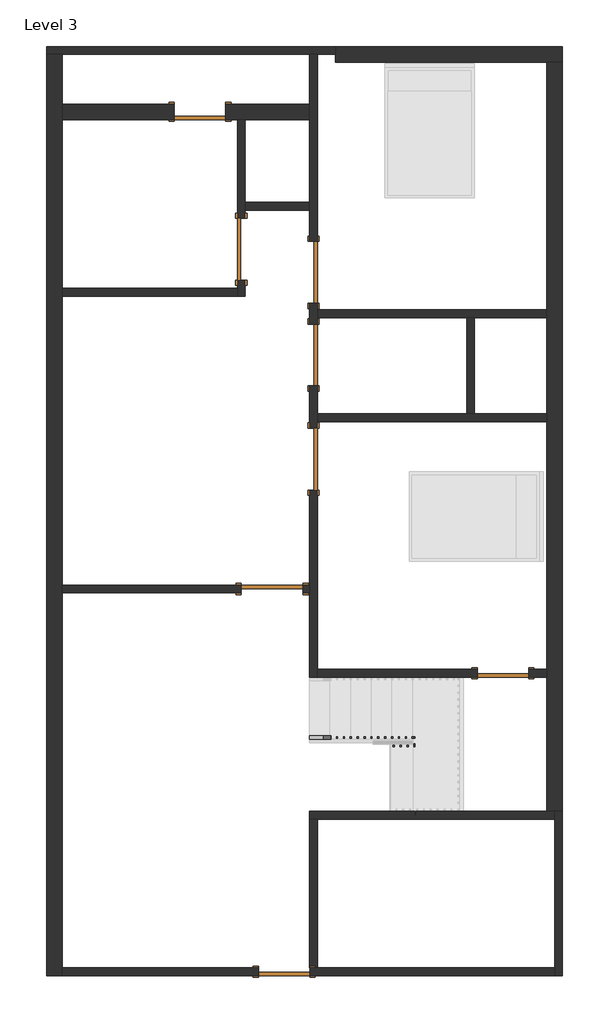
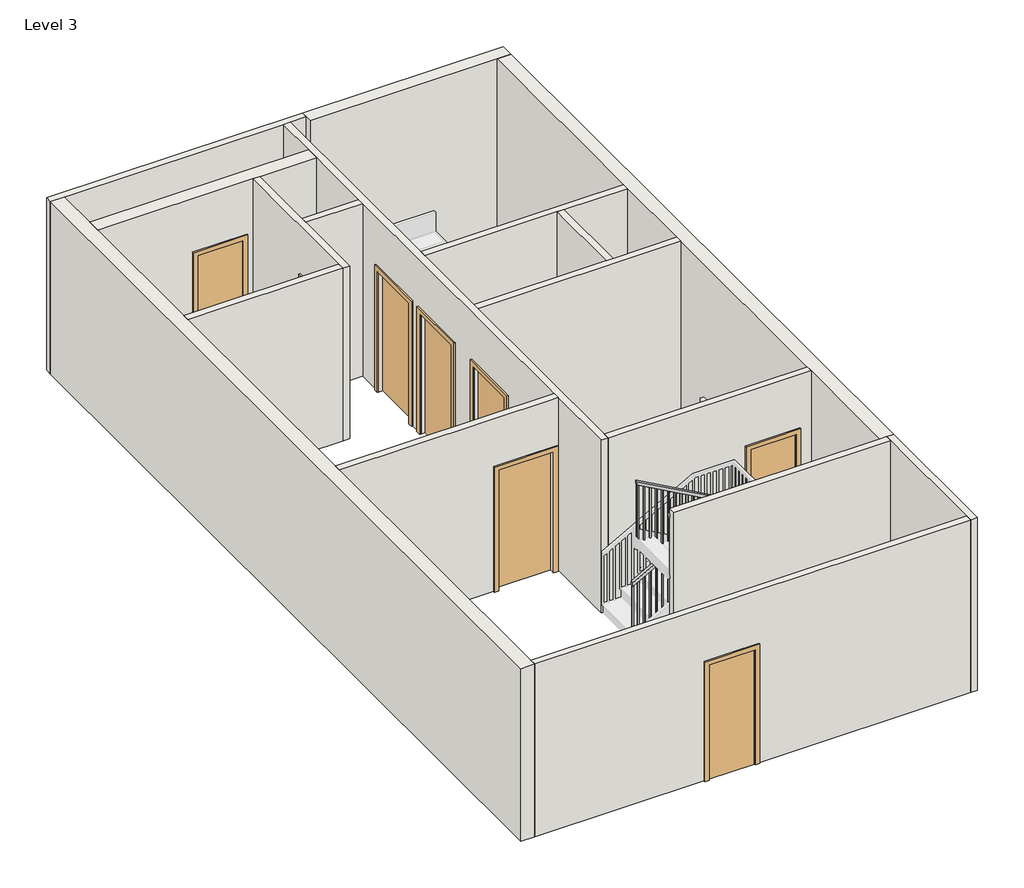
# One storey, part 1 of 2: 18 walls, 8 doors, 1 railing.
"""IFC4 building model written with IfcOpenShell, lengths in millimetres."""

from ifc_helpers import new_model, si_unit, frame, origin, place, context, project, spatial, polyline, outline, extrude, faceted_brep, transform, mapped, element, save
from components import door_85036156, door_d8f5dbb5, door_305aa2a5, door_e5f9f3c4

model = new_model("IFC4")

# Units and contexts
model_context = context("Model", 3, world=origin())
ifc_project = project(units=[si_unit("LENGTHUNIT", "METRE", prefix="MILLI")], contexts=[model_context])

# Site, building, storey
site = spatial("IfcSite", under=ifc_project)
building = spatial("IfcBuilding", under=site)
storey = spatial("IfcBuildingStorey", under=building, Name="Level 3", Elevation=3200.4)

# Doors
placement = place(None, origin())
door_shape = door_85036156(model_context)
element("IfcDoor", 1, ObjectType="Single-Flush : 30\" x 80\"", at=placement, inside=storey, context=model_context, shape_type="MappedRepresentation", body=[
    mapped(door_shape, transform((-2798.2915084, 6430.9935985, 3200.4), x_axis=(1.0, 0.0, 0.0), y_axis=(0.0, 1.0, 0.0), z_axis=(0.0, 0.0, 1.0))),
])
door_2_shape = door_d8f5dbb5(model_context)
element("IfcDoor", 2, ObjectType="Single-Flush : 30\" x 80\"", at=placement, inside=storey, context=model_context, shape_type="MappedRepresentation", body=[
    mapped(door_2_shape, transform((1678.4584916, -1855.7564015, 3200.4), x_axis=(-1.0, 0.0, 0.0), y_axis=(0.0, -1.0, 0.0), z_axis=(0.0, 0.0, 1.0))),
])
element("IfcDoor", 3, ObjectType="Single-Flush : 30\" x 80\"", at=placement, inside=storey, context=model_context, shape_type="MappedRepresentation", body=[
    mapped(door_2_shape, transform((-1553.6915084, -6262.6564015, 3200.4), x_axis=(-1.0, 0.0, 0.0), y_axis=(0.0, -1.0, 0.0), z_axis=(0.0, 0.0, 1.0))),
])
door_3_shape = door_305aa2a5(model_context)
element("IfcDoor", 4, ObjectType="Single-Flush : 36\" x 84\"", at=placement, inside=storey, context=model_context, shape_type="MappedRepresentation", body=[
    mapped(door_3_shape, transform((-2188.6915084, 4405.3435985, 3200.4), x_axis=(0.0, -1.0, 0.0), y_axis=(1.0, 0.0, 0.0), z_axis=(0.0, 0.0, 1.0))),
])
element("IfcDoor", 5, ObjectType="Single-Flush : 36\" x 84\"", at=placement, inside=storey, context=model_context, shape_type="MappedRepresentation", body=[
    mapped(door_3_shape, transform((-1121.8915084, 1306.5435985, 3200.4), x_axis=(0.0, 1.0, 0.0), y_axis=(-1.0, 0.0, 0.0), z_axis=(0.0, 0.0, 1.0))),
])
door_4_shape = door_e5f9f3c4(model_context)
element("IfcDoor", 6, ObjectType="Single-Flush : 36\" x 84\"", at=placement, inside=storey, context=model_context, shape_type="MappedRepresentation", body=[
    mapped(door_4_shape, transform((-1121.8915084, 4062.4435985, 3200.4), x_axis=(0.0, -1.0, 0.0), y_axis=(1.0, 0.0, 0.0), z_axis=(0.0, 0.0, 1.0))),
])
element("IfcDoor", 7, ObjectType="Single-Flush : 36\" x 84\"", at=placement, inside=storey, context=model_context, shape_type="MappedRepresentation", body=[
    mapped(door_4_shape, transform((-1121.8915084, 2843.2435985, 3200.4), x_axis=(0.0, -1.0, 0.0), y_axis=(1.0, 0.0, 0.0), z_axis=(0.0, 0.0, 1.0))),
])
element("IfcDoor", 8, ObjectType="Single-Flush : 36\" x 84\"", at=placement, inside=storey, context=model_context, shape_type="MappedRepresentation", body=[
    mapped(door_4_shape, transform((-1731.4915084, -611.1564015, 3200.4), x_axis=(1.0, 0.0, 0.0), y_axis=(0.0, 1.0, 0.0), z_axis=(0.0, 0.0, 1.0))),
])

# Railing
element("IfcRailing", 9, ObjectType="Handrail - Rectangular", at=placement, inside=storey, context=model_context, shape_type="SolidModel", body=[
    faceted_brep([(-1179.0415084, -2776.5064015, 4284.1333333), (-1179.0415084, -2776.5064015, 4226.020221), (-1179.0415084, -2827.3064015, 4226.020221), (-1179.0415084, -2827.3064015, 4284.1333333), (268.7584916, -2776.5064015, 5088.4666667), (319.5584916, -2776.5064015, 5058.5757765), (319.5584916, -2827.3064015, 5058.5757765), (268.7584916, -2827.3064015, 5088.4666667), (268.7584916, -2776.5064015, 5130.8), (319.5584916, -2776.5064015, 5080.0), (319.5584916, -2827.3064015, 5080.0), (268.7584916, -2827.3064015, 5130.8), (395.7584916, -2776.5064015, 5130.8), (395.7584916, -2776.5064015, 5080.0), (344.9584916, -2827.3064015, 5080.0), (344.9584916, -2827.3064015, 5130.8), (395.7584916, -2903.5064015, 5130.8), (395.7584916, -2903.5064015, 5080.0), (344.9584916, -2903.5064015, 5080.0), (344.9584916, -2903.5064015, 5130.8), (395.7584916, -2928.9064015, 5130.8), (344.9584916, -2928.9064015, 5130.8), (344.9584916, -2928.9064015, 5080.0), (395.7584916, -2928.9064015, 5080.0)], [[[0, 1, 2, 3]], [[1, 0, 4, 5]], [[2, 1, 5, 6]], [[3, 2, 6, 7]], [[0, 3, 7, 4]], [[5, 4, 8, 9]], [[6, 5, 9, 10]], [[7, 6, 10, 11]], [[4, 7, 11, 8]], [[9, 8, 12, 13]], [[10, 9, 13, 14]], [[11, 10, 14, 15]], [[8, 11, 15, 12]], [[13, 12, 16, 17]], [[14, 13, 17, 18]], [[15, 14, 18, 19]], [[12, 15, 19, 16]], [[20, 21, 22, 23]], [[17, 16, 20, 23]], [[18, 17, 23, 22]], [[19, 18, 22, 21]], [[16, 19, 21, 20]]]),
    faceted_brep([(395.7584916, -2903.5064015, 5130.8), (395.7584916, -2954.3064015, 5080.0), (344.9584916, -2954.3064015, 5080.0), (344.9584916, -2903.5064015, 5130.8), (395.7584916, -2903.5064015, 5271.9111111), (344.9584916, -2903.5064015, 5242.020221), (344.9584916, -2954.3064015, 5242.020221), (395.7584916, -2954.3064015, 5271.9111111)], [[[0, 1, 2, 3]], [[4, 5, 6, 7]], [[1, 0, 4, 7]], [[2, 1, 7, 6]], [[3, 2, 6, 5]], [[0, 3, 5, 4]]]),
    faceted_brep([(395.7584916, -2954.3064015, 5271.9111111), (344.9584916, -2954.3064015, 5242.020221), (344.9584916, -2903.5064015, 5242.020221), (395.7584916, -2903.5064015, 5271.9111111), (-1179.0415084, -2954.3064015, 6146.8), (-1179.0415084, -2903.5064015, 6146.8), (-1179.0415084, -2903.5064015, 6088.6868876), (-1179.0415084, -2954.3064015, 6088.6868876)], [[[0, 1, 2, 3]], [[4, 5, 6, 7]], [[1, 0, 4, 7]], [[2, 1, 7, 6]], [[3, 2, 6, 5]], [[0, 3, 5, 4]]]),
    extrude(outline(polyline([(6069.2841099, -1144.1165084), (6079.8674432, -1163.1665084), (5063.0666667, -1163.1665084), (5063.0666667, -1144.1165084), (6069.2841099, -1144.1165084)])), frame((0.0, -2938.4314015, 0.0), z_axis=(0.0, 1.0, 0.0), x_axis=(0.0, 0.0, 1.0)), (0.0, 0.0, 1.0), 19.05),
    extrude(outline(polyline([(6012.8396654, -1042.5165084), (6023.4229988, -1061.5665084), (5063.0666667, -1061.5665084), (5063.0666667, -1042.5165084), (6012.8396654, -1042.5165084)])), frame((0.0, -2938.4314015, 0.0), z_axis=(0.0, 1.0, 0.0), x_axis=(0.0, 0.0, 1.0)), (0.0, 0.0, 1.0), 19.05),
    extrude(outline(polyline([(5956.395221, -940.9165084), (5966.9785543, -959.9665084), (5063.0666667, -959.9665084), (5063.0666667, -940.9165084), (5956.395221, -940.9165084)])), frame((0.0, -2938.4314015, 0.0), z_axis=(0.0, 1.0, 0.0), x_axis=(0.0, 0.0, 1.0)), (0.0, 0.0, 1.0), 19.05),
    extrude(outline(polyline([(5899.9507765, -839.3165084), (5910.5341099, -858.3665084), (4893.7333333, -858.3665084), (4893.7333333, -839.3165084), (5899.9507765, -839.3165084)])), frame((0.0, -2938.4314015, 0.0), z_axis=(0.0, 1.0, 0.0), x_axis=(0.0, 0.0, 1.0)), (0.0, 0.0, 1.0), 19.05),
    extrude(outline(polyline([(5843.5063321, -737.7165084), (5854.0896654, -756.7665084), (4893.7333333, -756.7665084), (4893.7333333, -737.7165084), (5843.5063321, -737.7165084)])), frame((0.0, -2938.4314015, 0.0), z_axis=(0.0, 1.0, 0.0), x_axis=(0.0, 0.0, 1.0)), (0.0, 0.0, 1.0), 19.05),
    extrude(outline(polyline([(5787.0618876, -636.1165084), (5797.645221, -655.1665084), (4893.7333333, -655.1665084), (4893.7333333, -636.1165084), (5787.0618876, -636.1165084)])), frame((0.0, -2938.4314015, 0.0), z_axis=(0.0, 1.0, 0.0), x_axis=(0.0, 0.0, 1.0)), (0.0, 0.0, 1.0), 19.05),
    extrude(outline(polyline([(5730.6174432, -534.5165084), (5741.2007765, -553.5665084), (4724.4, -553.5665084), (4724.4, -534.5165084), (5730.6174432, -534.5165084)])), frame((0.0, -2938.4314015, 0.0), z_axis=(0.0, 1.0, 0.0), x_axis=(0.0, 0.0, 1.0)), (0.0, 0.0, 1.0), 19.05),
    extrude(outline(polyline([(5674.1729988, -432.9165084), (5684.7563321, -451.9665084), (4724.4, -451.9665084), (4724.4, -432.9165084), (5674.1729988, -432.9165084)])), frame((0.0, -2938.4314015, 0.0), z_axis=(0.0, 1.0, 0.0), x_axis=(0.0, 0.0, 1.0)), (0.0, 0.0, 1.0), 19.05),
    extrude(outline(polyline([(5617.7285543, -331.3165084), (5628.3118876, -350.3665084), (4724.4, -350.3665084), (4724.4, -331.3165084), (5617.7285543, -331.3165084)])), frame((0.0, -2938.4314015, 0.0), z_axis=(0.0, 1.0, 0.0), x_axis=(0.0, 0.0, 1.0)), (0.0, 0.0, 1.0), 19.05),
    extrude(outline(polyline([(5561.2841099, -229.7165084), (5571.8674432, -248.7665084), (4555.0666667, -248.7665084), (4555.0666667, -229.7165084), (5561.2841099, -229.7165084)])), frame((0.0, -2938.4314015, 0.0), z_axis=(0.0, 1.0, 0.0), x_axis=(0.0, 0.0, 1.0)), (0.0, 0.0, 1.0), 19.05),
    extrude(outline(polyline([(5504.8396654, -128.1165084), (5515.4229988, -147.1665084), (4555.0666667, -147.1665084), (4555.0666667, -128.1165084), (5504.8396654, -128.1165084)])), frame((0.0, -2938.4314015, 0.0), z_axis=(0.0, 1.0, 0.0), x_axis=(0.0, 0.0, 1.0)), (0.0, 0.0, 1.0), 19.05),
    extrude(outline(polyline([(5448.395221, -26.5165084), (5458.9785543, -45.5665084), (4555.0666667, -45.5665084), (4555.0666667, -26.5165084), (5448.395221, -26.5165084)])), frame((0.0, -2938.4314015, 0.0), z_axis=(0.0, 1.0, 0.0), x_axis=(0.0, 0.0, 1.0)), (0.0, 0.0, 1.0), 19.05),
    extrude(outline(polyline([(5391.9507765, 75.0834916), (5402.5341099, 56.0334916), (4385.7333333, 56.0334916), (4385.7333333, 75.0834916), (5391.9507765, 75.0834916)])), frame((0.0, -2938.4314015, 0.0), z_axis=(0.0, 1.0, 0.0), x_axis=(0.0, 0.0, 1.0)), (0.0, 0.0, 1.0), 19.05),
    extrude(outline(polyline([(5335.5063321, 176.6834916), (5346.0896654, 157.6334916), (4385.7333333, 157.6334916), (4385.7333333, 176.6834916), (5335.5063321, 176.6834916)])), frame((0.0, -2938.4314015, 0.0), z_axis=(0.0, 1.0, 0.0), x_axis=(0.0, 0.0, 1.0)), (0.0, 0.0, 1.0), 19.05),
    extrude(outline(polyline([(5279.0618876, 278.2834916), (5289.645221, 259.2334916), (4385.7333333, 259.2334916), (4385.7333333, 278.2834916), (5279.0618876, 278.2834916)])), frame((0.0, -2938.4314015, 0.0), z_axis=(0.0, 1.0, 0.0), x_axis=(0.0, 0.0, 1.0)), (0.0, 0.0, 1.0), 19.05),
    extrude(outline(polyline([(360.8334916, -2893.9814015), (379.8834916, -2893.9814015), (379.8834916, -2913.0314015), (360.8334916, -2913.0314015), (360.8334916, -2893.9814015)])), frame((0.0, 0.0, 4216.4), z_axis=(0.0, 0.0, 1.0), x_axis=(1.0, 0.0, 0.0)), (0.0, 0.0, 1.0), 863.6),
    extrude(outline(polyline([(335.4334916, -2811.4314015), (335.4334916, -2792.3814015), (354.4834916, -2792.3814015), (354.4834916, -2811.4314015), (335.4334916, -2811.4314015)])), frame((0.0, 0.0, 4216.4), z_axis=(0.0, 0.0, 1.0), x_axis=(1.0, 0.0, 0.0)), (0.0, 0.0, 1.0), 863.6),
    extrude(outline(polyline([(5021.5341099, 252.8834916), (5010.9507765, 233.8334916), (4047.0666667, 233.8334916), (4047.0666667, 252.8834916), (5021.5341099, 252.8834916)])), frame((0.0, -2811.4314015, 0.0), z_axis=(0.0, 1.0, 0.0), x_axis=(0.0, 0.0, 1.0)), (0.0, 0.0, 1.0), 19.05),
    extrude(outline(polyline([(4965.0896654, 151.2834916), (4954.5063321, 132.2334916), (4047.0666667, 132.2334916), (4047.0666667, 151.2834916), (4965.0896654, 151.2834916)])), frame((0.0, -2811.4314015, 0.0), z_axis=(0.0, 1.0, 0.0), x_axis=(0.0, 0.0, 1.0)), (0.0, 0.0, 1.0), 19.05),
    extrude(outline(polyline([(4908.645221, 49.6834916), (4898.0618876, 30.6334916), (4047.0666667, 30.6334916), (4047.0666667, 49.6834916), (4908.645221, 49.6834916)])), frame((0.0, -2811.4314015, 0.0), z_axis=(0.0, 1.0, 0.0), x_axis=(0.0, 0.0, 1.0)), (0.0, 0.0, 1.0), 19.05),
    extrude(outline(polyline([(4852.2007765, -51.9165084), (4841.6174432, -70.9665084), (3877.7333333, -70.9665084), (3877.7333333, -51.9165084), (4852.2007765, -51.9165084)])), frame((0.0, -2811.4314015, 0.0), z_axis=(0.0, 1.0, 0.0), x_axis=(0.0, 0.0, 1.0)), (0.0, 0.0, 1.0), 19.05),
    extrude(outline(polyline([(4795.7563321, -153.5165084), (4785.1729988, -172.5665084), (3877.7333333, -172.5665084), (3877.7333333, -153.5165084), (4795.7563321, -153.5165084)])), frame((0.0, -2811.4314015, 0.0), z_axis=(0.0, 1.0, 0.0), x_axis=(0.0, 0.0, 1.0)), (0.0, 0.0, 1.0), 19.05),
    extrude(outline(polyline([(4739.3118876, -255.1165084), (4728.7285543, -274.1665084), (3877.7333333, -274.1665084), (3877.7333333, -255.1165084), (4739.3118876, -255.1165084)])), frame((0.0, -2811.4314015, 0.0), z_axis=(0.0, 1.0, 0.0), x_axis=(0.0, 0.0, 1.0)), (0.0, 0.0, 1.0), 19.05),
    extrude(outline(polyline([(4682.8674432, -356.7165084), (4672.2841099, -375.7665084), (3708.4, -375.7665084), (3708.4, -356.7165084), (4682.8674432, -356.7165084)])), frame((0.0, -2811.4314015, 0.0), z_axis=(0.0, 1.0, 0.0), x_axis=(0.0, 0.0, 1.0)), (0.0, 0.0, 1.0), 19.05),
    extrude(outline(polyline([(4626.4229988, -458.3165084), (4615.8396654, -477.3665084), (3708.4, -477.3665084), (3708.4, -458.3165084), (4626.4229988, -458.3165084)])), frame((0.0, -2811.4314015, 0.0), z_axis=(0.0, 1.0, 0.0), x_axis=(0.0, 0.0, 1.0)), (0.0, 0.0, 1.0), 19.05),
    extrude(outline(polyline([(4569.9785543, -559.9165084), (4559.395221, -578.9665084), (3708.4, -578.9665084), (3708.4, -559.9165084), (4569.9785543, -559.9165084)])), frame((0.0, -2811.4314015, 0.0), z_axis=(0.0, 1.0, 0.0), x_axis=(0.0, 0.0, 1.0)), (0.0, 0.0, 1.0), 19.05),
    extrude(outline(polyline([(4513.5341099, -661.5165084), (4502.9507765, -680.5665084), (3539.0666667, -680.5665084), (3539.0666667, -661.5165084), (4513.5341099, -661.5165084)])), frame((0.0, -2811.4314015, 0.0), z_axis=(0.0, 1.0, 0.0), x_axis=(0.0, 0.0, 1.0)), (0.0, 0.0, 1.0), 19.05),
    extrude(outline(polyline([(4457.0896654, -763.1165084), (4446.5063321, -782.1665084), (3539.0666667, -782.1665084), (3539.0666667, -763.1165084), (4457.0896654, -763.1165084)])), frame((0.0, -2811.4314015, 0.0), z_axis=(0.0, 1.0, 0.0), x_axis=(0.0, 0.0, 1.0)), (0.0, 0.0, 1.0), 19.05),
    extrude(outline(polyline([(4400.645221, -864.7165084), (4390.0618876, -883.7665084), (3539.0666667, -883.7665084), (3539.0666667, -864.7165084), (4400.645221, -864.7165084)])), frame((0.0, -2811.4314015, 0.0), z_axis=(0.0, 1.0, 0.0), x_axis=(0.0, 0.0, 1.0)), (0.0, 0.0, 1.0), 19.05),
    extrude(outline(polyline([(4344.2007765, -966.3165084), (4333.6174432, -985.3665084), (3369.7333333, -985.3665084), (3369.7333333, -966.3165084), (4344.2007765, -966.3165084)])), frame((0.0, -2811.4314015, 0.0), z_axis=(0.0, 1.0, 0.0), x_axis=(0.0, 0.0, 1.0)), (0.0, 0.0, 1.0), 19.05),
    extrude(outline(polyline([(4287.7563321, -1067.9165084), (4277.1729988, -1086.9665084), (3369.7333333, -1086.9665084), (3369.7333333, -1067.9165084), (4287.7563321, -1067.9165084)])), frame((0.0, -2811.4314015, 0.0), z_axis=(0.0, 1.0, 0.0), x_axis=(0.0, 0.0, 1.0)), (0.0, 0.0, 1.0), 19.05),
    extrude(outline(polyline([(360.8334916, -2919.3814015), (379.8834916, -2919.3814015), (379.8834916, -2938.4314015), (360.8334916, -2938.4314015), (360.8334916, -2919.3814015)])), frame((0.0, 0.0, 4216.4), z_axis=(0.0, 0.0, 1.0), x_axis=(1.0, 0.0, 0.0)), (0.0, 0.0, 1.0), 863.6),
    extrude(outline(polyline([(360.8334916, -2811.4314015), (360.8334916, -2792.3814015), (379.8834916, -2792.3814015), (379.8834916, -2811.4314015), (360.8334916, -2811.4314015)])), frame((0.0, 0.0, 4216.4), z_axis=(0.0, 0.0, 1.0), x_axis=(1.0, 0.0, 0.0)), (0.0, 0.0, 1.0), 863.6),
    extrude(outline(polyline([(6078.1035543, -1159.9915084), (6088.6868876, -1179.0415084), (5063.0666667, -1179.0415084), (5063.0666667, -1159.9915084), (6078.1035543, -1159.9915084)])), frame((0.0, -2938.4314015, 0.0), z_axis=(0.0, 1.0, 0.0), x_axis=(0.0, 0.0, 1.0)), (0.0, 0.0, 1.0), 19.05),
    extrude(outline(polyline([(4236.6035543, -1159.9915084), (4226.020221, -1179.0415084), (3369.7333333, -1179.0415084), (3369.7333333, -1159.9915084), (4236.6035543, -1159.9915084)])), frame((0.0, -2811.4314015, 0.0), z_axis=(0.0, 1.0, 0.0), x_axis=(0.0, 0.0, 1.0)), (0.0, 0.0, 1.0), 19.05),
])

# Walls
element("IfcWall", 10, ObjectType="WALL 9\"", at=placement, inside=storey, context=model_context, shape_type="Brep", body=[
    faceted_brep([(-798.0415084, 7167.5935985, 3200.4), (2326.1584916, 7167.5935985, 3200.4), (2554.7584916, 7167.5935985, 3200.4), (2554.7584916, 7167.5935985, 6248.4), (2326.1584916, 7167.5935985, 6248.4), (-798.0415084, 7167.5935985, 6248.4), (-798.0415084, 7396.1935985, 3200.4), (-798.0415084, 7396.1935985, 6248.4), (2554.7584916, 7396.1935985, 6248.4), (2554.7584916, 7396.1935985, 3200.4), (-798.0415084, 7281.8935985, 3200.4), (-798.0415084, 7281.8935985, 6248.4)], [[[0, 1, 2, 3, 4, 5]], [[6, 7, 8, 9]], [[2, 1, 0, 10, 6, 9]], [[0, 5, 11, 7, 6, 10]], [[3, 2, 9, 8]], [[5, 4, 3, 8, 7, 11]]]),
])
element("IfcWall", 11, ObjectType="WALL 9\"", at=placement, inside=storey, context=model_context, shape_type="Brep", body=[
    faceted_brep([(2326.1584916, 7167.5935985, 3200.4), (2326.1584916, 3509.9935985, 3200.4), (2326.1584916, 3395.6935985, 3200.4), (2326.1584916, 1973.2935985, 3200.4), (2326.1584916, 1858.9935985, 3200.4), (2326.1584916, -1798.6064015, 3200.4), (2326.1584916, -1912.9064015, 3200.4), (2326.1584916, -3894.1064015, 3200.4), (2326.1584916, -3894.1064015, 6248.4), (2326.1584916, -1912.9064015, 6248.4), (2326.1584916, -1798.6064015, 6248.4), (2326.1584916, 1858.9935985, 6248.4), (2326.1584916, 1973.2935985, 6248.4), (2326.1584916, 3395.6935985, 6248.4), (2326.1584916, 3509.9935985, 6248.4), (2326.1584916, 7167.5935985, 6248.4), (2554.7584916, 7167.5935985, 3200.4), (2554.7584916, 7167.5935985, 6248.4), (2554.7584916, -3894.1064015, 6248.4), (2554.7584916, -3894.1064015, 3200.4), (2440.4584916, -3894.1064015, 3200.4), (2440.4584916, -3894.1064015, 6248.4)], [[[0, 1, 2, 3, 4, 5, 6, 7, 8, 9, 10, 11, 12, 13, 14, 15]], [[16, 17, 18, 19]], [[7, 6, 5, 4, 3, 2, 1, 0, 16, 19, 20]], [[0, 15, 17, 16]], [[8, 7, 20, 19, 18, 21]], [[15, 14, 13, 12, 11, 10, 9, 8, 21, 18, 17]]]),
])
element("IfcWall", 12, ObjectType="WALL 9\"", at=placement, inside=storey, context=model_context, shape_type="Brep", body=[
    faceted_brep([(-5065.2415084, 7281.8935985, 3200.4), (-5065.2415084, -6319.8064015, 3200.4), (-5065.2415084, -6319.8064015, 6248.4), (-5065.2415084, 7281.8935985, 6248.4), (-4836.6415084, 7281.8935985, 3200.4), (-4836.6415084, 7281.8935985, 6248.4), (-4836.6415084, 6545.2935985, 6248.4), (-4836.6415084, 6316.6935985, 6248.4), (-4836.6415084, 3827.4935985, 6248.4), (-4836.6415084, 3713.1935985, 6248.4), (-4836.6415084, -554.0064015, 6248.4), (-4836.6415084, -668.3064015, 6248.4), (-4836.6415084, -6205.5064015, 6248.4), (-4836.6415084, -6319.8064015, 6248.4), (-4836.6415084, -6319.8064015, 3200.4), (-4836.6415084, -6205.5064015, 3200.4), (-4836.6415084, -668.3064015, 3200.4), (-4836.6415084, -554.0064015, 3200.4), (-4836.6415084, 3713.1935985, 3200.4), (-4836.6415084, 3827.4935985, 3200.4), (-4836.6415084, 6316.6935985, 3200.4), (-4836.6415084, 6545.2935985, 3200.4)], [[[0, 1, 2, 3]], [[4, 5, 6, 7, 8, 9, 10, 11, 12, 13, 14, 15, 16, 17, 18, 19, 20, 21]], [[1, 0, 4, 21, 20, 19, 18, 17, 16, 15, 14]], [[0, 3, 5, 4]], [[3, 2, 13, 12, 11, 10, 9, 8, 7, 6, 5]], [[2, 1, 14, 13]]]),
])
element("IfcWall", 13, ObjectType="WALL 9\"", at=placement, inside=storey, context=model_context, shape_type="Brep", body=[
    faceted_brep([(-2417.2915084, 6316.6935985, 5232.4), (-2417.2915084, 6316.6935985, 3200.4), (-2245.8415084, 6316.6935985, 3200.4), (-2131.5415084, 6316.6935985, 3200.4), (-1179.0415084, 6316.6935985, 3200.4), (-1179.0415084, 6316.6935985, 6248.4), (-2131.5415084, 6316.6935985, 6248.4), (-2245.8415084, 6316.6935985, 6248.4), (-4836.6415084, 6316.6935985, 6248.4), (-4836.6415084, 6316.6935985, 3200.4), (-3179.2915084, 6316.6935985, 3200.4), (-3179.2915084, 6316.6935985, 5232.4), (-1179.0415084, 6545.2935985, 3200.4), (-2417.2915084, 6545.2935985, 3200.4), (-2417.2915084, 6545.2935985, 5232.4), (-3179.2915084, 6545.2935985, 5232.4), (-3179.2915084, 6545.2935985, 3200.4), (-4836.6415084, 6545.2935985, 3200.4), (-4836.6415084, 6545.2935985, 6248.4), (-1179.0415084, 6545.2935985, 6248.4)], [[[0, 1, 2, 3, 4, 5, 6, 7, 8, 9, 10, 11]], [[12, 13, 14, 15, 16, 17, 18, 19]], [[10, 9, 17, 16]], [[4, 3, 2, 1, 13, 12]], [[9, 8, 18, 17]], [[5, 4, 12, 19]], [[14, 13, 1, 0]], [[15, 14, 0, 11]], [[16, 15, 11, 10]], [[8, 7, 6, 5, 19, 18]]]),
])
element("IfcWall", 14, ObjectType="WALL4.5\"", at=placement, inside=storey, context=model_context, shape_type="Brep", body=[
    faceted_brep([(-5065.2415084, 7281.8935985, 3200.4), (-4836.6415084, 7281.8935985, 3200.4), (-1179.0415084, 7281.8935985, 3200.4), (-1064.7415084, 7281.8935985, 3200.4), (-798.0415084, 7281.8935985, 3200.4), (-798.0415084, 7281.8935985, 6248.4), (-1064.7415084, 7281.8935985, 6248.4), (-1179.0415084, 7281.8935985, 6248.4), (-4836.6415084, 7281.8935985, 6248.4), (-5065.2415084, 7281.8935985, 6248.4), (-5065.2415084, 7396.1935985, 3200.4), (-5065.2415084, 7396.1935985, 6248.4), (-798.0415084, 7396.1935985, 6248.4), (-798.0415084, 7396.1935985, 3200.4)], [[[0, 1, 2, 3, 4, 5, 6, 7, 8, 9]], [[10, 11, 12, 13]], [[4, 3, 2, 1, 0, 10, 13]], [[5, 4, 13, 12]], [[0, 9, 11, 10]], [[9, 8, 7, 6, 5, 12, 11]]]),
])
element("IfcWall", 15, ObjectType="WALL4.5\"", at=placement, inside=storey, context=model_context, shape_type="Brep", body=[
    faceted_brep([(2554.7584916, -6319.8064015, 3200.4), (2554.7584916, -3894.1064015, 3200.4), (2554.7584916, -3894.1064015, 6248.4), (2554.7584916, -6319.8064015, 6248.4), (2440.4584916, -6319.8064015, 3200.4), (2440.4584916, -6319.8064015, 6248.4), (2440.4584916, -6205.5064015, 6248.4), (2440.4584916, -4008.4064015, 6248.4), (2440.4584916, -3894.1064015, 6248.4), (2440.4584916, -3894.1064015, 3200.4), (2440.4584916, -4008.4064015, 3200.4), (2440.4584916, -6205.5064015, 3200.4)], [[[0, 1, 2, 3]], [[4, 5, 6, 7, 8, 9, 10, 11]], [[1, 0, 4, 11, 10, 9]], [[3, 2, 8, 7, 6, 5]], [[2, 1, 9, 8]], [[0, 3, 5, 4]]]),
])
element("IfcWall", 16, ObjectType="WALL4.5\"", at=placement, inside=storey, context=model_context, shape_type="Brep", body=[
    faceted_brep([(2440.4584916, -3894.1064015, 3200.4), (2326.1584916, -3894.1064015, 3200.4), (-1179.0415084, -3894.1064015, 3200.4), (-1179.0415084, -3894.1064015, 6248.4), (2326.1584916, -3894.1064015, 6248.4), (2440.4584916, -3894.1064015, 6248.4), (2440.4584916, -4008.4064015, 3200.4), (2440.4584916, -4008.4064015, 6248.4), (-1179.0415084, -4008.4064015, 6248.4), (-1179.0415084, -4008.4064015, 4419.6), (-1179.0415084, -4008.4064015, 3200.4), (-1064.7415084, -4008.4064015, 3200.4)], [[[0, 1, 2, 3, 4, 5]], [[6, 7, 8, 9, 10, 11]], [[2, 1, 0, 6, 11, 10]], [[0, 5, 7, 6]], [[3, 2, 10, 9, 8]], [[5, 4, 3, 8, 7]]]),
])
element("IfcWall", 17, ObjectType="WALL4.5\"", at=placement, inside=storey, context=model_context, shape_type="Brep", body=[
    faceted_brep([(-2245.8415084, 3948.1435985, 5334.0), (-2245.8415084, 3948.1435985, 3200.4), (-2245.8415084, 3827.4935985, 3200.4), (-2245.8415084, 3713.1935985, 3200.4), (-2245.8415084, 3713.1935985, 6248.4), (-2245.8415084, 3827.4935985, 6248.4), (-2245.8415084, 6316.6935985, 6248.4), (-2245.8415084, 6316.6935985, 3200.4), (-2245.8415084, 4862.5435985, 3200.4), (-2245.8415084, 4862.5435985, 5334.0), (-2131.5415084, 3713.1935985, 3200.4), (-2131.5415084, 3948.1435985, 3200.4), (-2131.5415084, 3948.1435985, 5334.0), (-2131.5415084, 4862.5435985, 5334.0), (-2131.5415084, 4862.5435985, 3200.4), (-2131.5415084, 4983.1935985, 3200.4), (-2131.5415084, 5097.4935985, 3200.4), (-2131.5415084, 6316.6935985, 3200.4), (-2131.5415084, 6316.6935985, 6248.4), (-2131.5415084, 5097.4935985, 6248.4), (-2131.5415084, 4983.1935985, 6248.4), (-2131.5415084, 3713.1935985, 6248.4)], [[[0, 1, 2, 3, 4, 5, 6, 7, 8, 9]], [[10, 11, 12, 13, 14, 15, 16, 17, 18, 19, 20, 21]], [[8, 7, 17, 16, 15, 14]], [[3, 2, 1, 11, 10]], [[7, 6, 18, 17]], [[4, 3, 10, 21]], [[12, 11, 1, 0]], [[13, 12, 0, 9]], [[14, 13, 9, 8]], [[6, 5, 4, 21, 20, 19, 18]]]),
])
element("IfcWall", 18, ObjectType="WALL4.5\"", at=placement, inside=storey, context=model_context, shape_type="SweptSolid", body=[
    extrude(outline(polyline([(-2245.8415084, 3713.1935985), (-4836.6415084, 3713.1935985), (-4836.6415084, 3827.4935985), (-2245.8415084, 3827.4935985), (-2245.8415084, 3713.1935985)])), frame((0.0, 0.0, 3200.4), z_axis=(0.0, 0.0, 1.0), x_axis=(1.0, 0.0, 0.0)), (0.0, 0.0, 1.0), 3048.0),
])
element("IfcWall", 19, ObjectType="WALL4.5\"", at=placement, inside=storey, context=model_context, shape_type="SweptSolid", body=[
    extrude(outline(polyline([(-1179.0415084, 4983.1935985), (-2131.5415084, 4983.1935985), (-2131.5415084, 5097.4935985), (-1179.0415084, 5097.4935985), (-1179.0415084, 4983.1935985)])), frame((0.0, 0.0, 3200.4), z_axis=(0.0, 0.0, 1.0), x_axis=(1.0, 0.0, 0.0)), (0.0, 0.0, 1.0), 3048.0),
])
element("IfcWall", 20, ObjectType="WALL4.5\"", at=placement, inside=storey, context=model_context, shape_type="Brep", body=[
    faceted_brep([(-1179.0415084, 2386.0435985, 3200.4), (-1179.0415084, 1763.7435985, 3200.4), (-1179.0415084, 1763.7435985, 5334.0), (-1179.0415084, 849.3435985, 5334.0), (-1179.0415084, 849.3435985, 3200.4), (-1179.0415084, -554.0064015, 3200.4), (-1179.0415084, -668.3064015, 3200.4), (-1179.0415084, -1912.9064015, 3200.4), (-1179.0415084, -1912.9064015, 6248.4), (-1179.0415084, -668.3064015, 6248.4), (-1179.0415084, -554.0064015, 6248.4), (-1179.0415084, 4983.1935985, 6248.4), (-1179.0415084, 5097.4935985, 6248.4), (-1179.0415084, 6316.6935985, 6248.4), (-1179.0415084, 6545.2935985, 6248.4), (-1179.0415084, 7281.8935985, 6248.4), (-1179.0415084, 7281.8935985, 3200.4), (-1179.0415084, 6545.2935985, 3200.4), (-1179.0415084, 6316.6935985, 3200.4), (-1179.0415084, 5097.4935985, 3200.4), (-1179.0415084, 4983.1935985, 3200.4), (-1179.0415084, 4519.6435985, 3200.4), (-1179.0415084, 4519.6435985, 5334.0), (-1179.0415084, 3605.2435985, 5334.0), (-1179.0415084, 3605.2435985, 3200.4), (-1179.0415084, 3300.4435985, 3200.4), (-1179.0415084, 3300.4435985, 5334.0), (-1179.0415084, 2386.0435985, 5334.0), (-1064.7415084, 1763.7435985, 5334.0), (-1064.7415084, 1763.7435985, 3200.4), (-1064.7415084, 1858.9935985, 3200.4), (-1064.7415084, 1973.2935985, 3200.4), (-1064.7415084, 2386.0435985, 3200.4), (-1064.7415084, 2386.0435985, 5334.0), (-1064.7415084, 3300.4435985, 5334.0), (-1064.7415084, 3300.4435985, 3200.4), (-1064.7415084, 3395.6935985, 3200.4), (-1064.7415084, 3509.9935985, 3200.4), (-1064.7415084, 3605.2435985, 3200.4), (-1064.7415084, 3605.2435985, 5334.0), (-1064.7415084, 4519.6435985, 5334.0), (-1064.7415084, 4519.6435985, 3200.4), (-1064.7415084, 7281.8935985, 3200.4), (-1064.7415084, 7281.8935985, 6248.4), (-1064.7415084, 3509.9935985, 6248.4), (-1064.7415084, 3395.6935985, 6248.4), (-1064.7415084, 1973.2935985, 6248.4), (-1064.7415084, 1858.9935985, 6248.4), (-1064.7415084, -1798.6064015, 6248.4), (-1064.7415084, -1912.9064015, 6248.4), (-1064.7415084, -1912.9064015, 3200.4), (-1064.7415084, -1798.6064015, 3200.4), (-1064.7415084, 849.3435985, 3200.4), (-1064.7415084, 849.3435985, 5334.0)], [[[0, 1, 2, 3, 4, 5, 6, 7, 8, 9, 10, 11, 12, 13, 14, 15, 16, 17, 18, 19, 20, 21, 22, 23, 24, 25, 26, 27]], [[28, 29, 30, 31, 32, 33, 34, 35, 36, 37, 38, 39, 40, 41, 42, 43, 44, 45, 46, 47, 48, 49, 50, 51, 52, 53]], [[21, 20, 19, 18, 17, 16, 42, 41]], [[25, 24, 38, 37, 36, 35]], [[52, 51, 50, 7, 6, 5, 4]], [[32, 31, 30, 29, 1, 0]], [[16, 15, 43, 42]], [[8, 7, 50, 49]], [[39, 38, 24, 23]], [[40, 39, 23, 22]], [[41, 40, 22, 21]], [[33, 32, 0, 27]], [[34, 33, 27, 26]], [[35, 34, 26, 25]], [[2, 1, 29, 28]], [[3, 2, 28, 53]], [[4, 3, 53, 52]], [[15, 14, 13, 12, 11, 10, 9, 8, 49, 48, 47, 46, 45, 44, 43]]]),
])
element("IfcWall", 21, ObjectType="WALL4.5\"", at=placement, inside=storey, context=model_context, shape_type="SweptSolid", body=[
    extrude(outline(polyline([(3200.4, -1064.7415084), (3200.4, 1297.4584916), (5232.4, 1297.4584916), (5232.4, 2059.4584916), (3200.4, 2059.4584916), (3200.4, 2326.1584916), (6248.4, 2326.1584916), (6248.4, -1064.7415084), (3200.4, -1064.7415084)])), frame((0.0, -1912.9064015, 0.0), z_axis=(0.0, 1.0, 0.0), x_axis=(0.0, 0.0, 1.0)), (0.0, 0.0, 1.0), 114.3),
])
element("IfcWall", 22, ObjectType="WALL4.5\"", at=placement, inside=storey, context=model_context, shape_type="Brep", body=[
    faceted_brep([(-1064.7415084, 3395.6935985, 3200.4), (1145.0584916, 3395.6935985, 3200.4), (1259.3584916, 3395.6935985, 3200.4), (2326.1584916, 3395.6935985, 3200.4), (2326.1584916, 3395.6935985, 6248.4), (1259.3584916, 3395.6935985, 6248.4), (1145.0584916, 3395.6935985, 6248.4), (-1064.7415084, 3395.6935985, 6248.4), (-1064.7415084, 3509.9935985, 3200.4), (-1064.7415084, 3509.9935985, 6248.4), (2326.1584916, 3509.9935985, 6248.4), (2326.1584916, 3509.9935985, 3200.4)], [[[0, 1, 2, 3, 4, 5, 6, 7]], [[8, 9, 10, 11]], [[3, 2, 1, 0, 8, 11]], [[4, 3, 11, 10]], [[0, 7, 9, 8]], [[7, 6, 5, 4, 10, 9]]]),
])
element("IfcWall", 23, ObjectType="WALL4.5\"", at=placement, inside=storey, context=model_context, shape_type="SweptSolid", body=[
    extrude(outline(polyline([(1259.3584916, 3395.6935985), (1259.3584916, 1973.2935985), (1145.0584916, 1973.2935985), (1145.0584916, 3395.6935985), (1259.3584916, 3395.6935985)])), frame((0.0, 0.0, 3200.4), z_axis=(0.0, 0.0, 1.0), x_axis=(1.0, 0.0, 0.0)), (0.0, 0.0, 1.0), 3048.0),
])
element("IfcWall", 24, ObjectType="WALL4.5\"", at=placement, inside=storey, context=model_context, shape_type="Brep", body=[
    faceted_brep([(-1064.7415084, 1858.9935985, 3200.4), (2326.1584916, 1858.9935985, 3200.4), (2326.1584916, 1858.9935985, 6248.4), (-1064.7415084, 1858.9935985, 6248.4), (-1064.7415084, 1973.2935985, 3200.4), (-1064.7415084, 1973.2935985, 6248.4), (1145.0584916, 1973.2935985, 6248.4), (1259.3584916, 1973.2935985, 6248.4), (2326.1584916, 1973.2935985, 6248.4), (2326.1584916, 1973.2935985, 3200.4), (1259.3584916, 1973.2935985, 3200.4), (1145.0584916, 1973.2935985, 3200.4)], [[[0, 1, 2, 3]], [[4, 5, 6, 7, 8, 9, 10, 11]], [[1, 0, 4, 11, 10, 9]], [[2, 1, 9, 8]], [[0, 3, 5, 4]], [[3, 2, 8, 7, 6, 5]]]),
])
element("IfcWall", 25, ObjectType="WALL4.5\"", at=placement, inside=storey, context=model_context, shape_type="SweptSolid", body=[
    extrude(outline(polyline([(5334.0, -1274.2915084), (3200.4, -1274.2915084), (3200.4, -1179.0415084), (6248.4, -1179.0415084), (6248.4, -4836.6415084), (3200.4, -4836.6415084), (3200.4, -2188.6915084), (5334.0, -2188.6915084), (5334.0, -1274.2915084)])), frame((0.0, -668.3064015, 0.0), z_axis=(0.0, 1.0, 0.0), x_axis=(0.0, 0.0, 1.0)), (0.0, 0.0, 1.0), 114.3),
])
element("IfcWall", 26, ObjectType="WALL4.5\"", at=placement, inside=storey, context=model_context, shape_type="SweptSolid", body=[
    extrude(outline(polyline([(-1179.0415084, -6205.5064015), (-1179.0415084, -4008.4064015), (-1064.7415084, -4008.4064015), (-1064.7415084, -6205.5064015), (-1179.0415084, -6205.5064015)])), frame((0.0, 0.0, 3200.4), z_axis=(0.0, 0.0, 1.0), x_axis=(1.0, 0.0, 0.0)), (0.0, 0.0, 1.0), 1219.2),
])
element("IfcWall", 27, ObjectType="WALL4.5\"", at=placement, inside=storey, context=model_context, shape_type="Brep", body=[
    faceted_brep([(-4836.6415084, -6319.8064015, 3200.4), (-1934.6915084, -6319.8064015, 3200.4), (-1934.6915084, -6319.8064015, 5232.4), (-1172.6915084, -6319.8064015, 5232.4), (-1172.6915084, -6319.8064015, 3200.4), (2440.4584916, -6319.8064015, 3200.4), (2440.4584916, -6319.8064015, 6248.4), (-4836.6415084, -6319.8064015, 6248.4), (-1934.6915084, -6205.5064015, 5232.4), (-1934.6915084, -6205.5064015, 3200.4), (-4836.6415084, -6205.5064015, 3200.4), (-4836.6415084, -6205.5064015, 6248.4), (2440.4584916, -6205.5064015, 6248.4), (2440.4584916, -6205.5064015, 3200.4), (-1064.7415084, -6205.5064015, 3200.4), (-1172.6915084, -6205.5064015, 3200.4), (-1172.6915084, -6205.5064015, 5232.4)], [[[0, 1, 2, 3, 4, 5, 6, 7]], [[8, 9, 10, 11, 12, 13, 14, 15, 16]], [[10, 9, 1, 0]], [[15, 14, 13, 5, 4]], [[7, 6, 12, 11]], [[0, 7, 11, 10]], [[6, 5, 13, 12]], [[2, 1, 9, 8]], [[3, 2, 8, 16]], [[4, 3, 16, 15]]]),
])

save(model, "model.ifc")

# Revit data of these elements
# Type "Single-Flush : 30\" x 80\""
#   Type Mark = "5"
#   Construction Type Id = "MDOOR"
#   Assembly Code = "C1020"
#   Analytic Construction = "Metal"
#   Thickness = 0' - 2"
#   Heat Transfer Coefficient (U) = 0.651978 BTU/(h·ft²·°F)
#   Height = 6' - 8"
#   Trim Projection Ext = 0' - 1"
#   Trim Projection Int = 0' - 1"
#   Trim Width = 0' - 3"
#   Width = 2' - 6"
#   Define Thermal Properties by = 1
#   Define Thermal Properties by = 1
#   Door Material = Door - Panel
#   Frame Material = Door - Frame
#   Visual Light Transmittance = 0
#   Solar Heat Gain Coefficient = 0
#   Function = (empty or 0)
#   Wall Closure = (empty or 0)
# Type "Single-Flush : 36\" x 84\""
#   Type Mark = "1"
#   Construction Type Id = "MDOOR"
#   Assembly Code = "C1020"
#   Analytic Construction = "Metal"
#   Thickness = 0' - 2"
#   Heat Transfer Coefficient (U) = 0.651978 BTU/(h·ft²·°F)
#   Height = 7' - 0"
#   Trim Projection Ext = 0' - 1"
#   Trim Projection Int = 0' - 1"
#   Trim Width = 0' - 3"
#   Width = 3' - 0"
#   Define Thermal Properties by = 1
#   Define Thermal Properties by = 1
#   Door Material = Door - Panel
#   Frame Material = Door - Frame
#   Visual Light Transmittance = 0
#   Solar Heat Gain Coefficient = 0
#   Function = (empty or 0)
#   Wall Closure = (empty or 0)
# Type "Handrail - Rectangular"
#   Assembly Code = "C2010400"
#   built-in parameter 1008612 = 0.0416667 (stored number, unit not read)
#   built-in parameter 1008611 = 0.0416667 (stored number, unit not read)
#   built-in parameter 1008609 = 0.333333 (stored number, unit not read)
#   built-in parameter 1008604 = 0.166667 (stored number, unit not read)
#   built-in parameter 1008603 = 0.166667 (stored number, unit not read)
#   Railing Height = 3' - 0"
#   built-in parameter 1008630 = 2
#   built-in parameter 1008610 = 2
#   built-in parameter 1008618 = Baluster - Square : 3/4"
# Type "WALL 9\""
#   Assembly Code = "B2010"
#   Layers, outside or top first: 0' - 9" no material (function 1)
# Type "WALL4.5\""
#   Assembly Code = "B2010"
#   Layers, outside or top first: 0' - 4 1/2" no material (function 1)
# Elements 1, 2, 3 (IfcDoor, "Single-Flush : 30\" x 80\"")
#   Phase Created = New Construction
#   Materials on its faces: "Door - Frame", "Door - Panel"
# Elements 4, 5, 6, 7, 8 (IfcDoor, "Single-Flush : 36\" x 84\"")
#   Phase Created = New Construction
#   Materials on its faces: "Door - Frame", "Door - Panel"
# Element 9 (IfcRailing, "Handrail - Rectangular")
#   Phase Created = New Construction
# Elements 10, 11, 12 (IfcWall, "WALL 9\"")
#   Top Offset = 0' - 0"
#   Base Offset = 0' - 0"
#   Unconnected Height = 10' - 0"
#   wall height = 10' - 0"
#   Phase Created = New Construction
#   Base Constraint = Level 3
#   Materials on its faces: "Default Wall", "Brick, Common"
# Element 13 (IfcWall, "WALL 9\"")
#   Top Offset = 0' - 0"
#   Base Offset = 0' - 0"
#   Unconnected Height = 10' - 0"
#   wall height = 10' - 0"
#   Phase Created = New Construction
#   Base Constraint = Level 3
#   Materials on its faces: "Default Wall"
# Elements 14, 15, 27 (IfcWall, "WALL4.5\"")
#   Top Offset = 0' - 0"
#   Base Offset = 0' - 0"
#   Unconnected Height = 10' - 0"
#   wall height = 10' - 0"
#   Phase Created = New Construction
#   Base Constraint = Level 3
#   Materials on its faces: "Default Wall", "Brick, Common"
# Elements 16, 17, 18, 19, 20, 21, 22, 23, 24, 25 (IfcWall, "WALL4.5\"")
#   Top Offset = 0' - 0"
#   Base Offset = 0' - 0"
#   Unconnected Height = 10' - 0"
#   wall height = 10' - 0"
#   Phase Created = New Construction
#   Base Constraint = Level 3
#   Materials on its faces: "Default Wall"
# Element 26 (IfcWall, "WALL4.5\"")
#   Top Offset = 0' - 0"
#   Base Offset = 0' - 0"
#   Unconnected Height = 4' - 0"
#   wall height = 4' - 0"
#   Phase Created = New Construction
#   Base Constraint = Level 3
#   Materials on its faces: "Default Wall"
# Materials
#   "Door - Panel": class "Wood", colour RGB 210 159 95, transparency 0, Cost = 0
#   "Door - Frame": colour RGB 118 70 51, transparency 0, Cost = 0
#   "Default Wall": colour RGB 128 128 128, transparency 0, Cost = 0
#   "Brick, Common": class "Masonry", colour RGB 170 98 104, transparency 0, Description = "Common brick", Cost = 0
